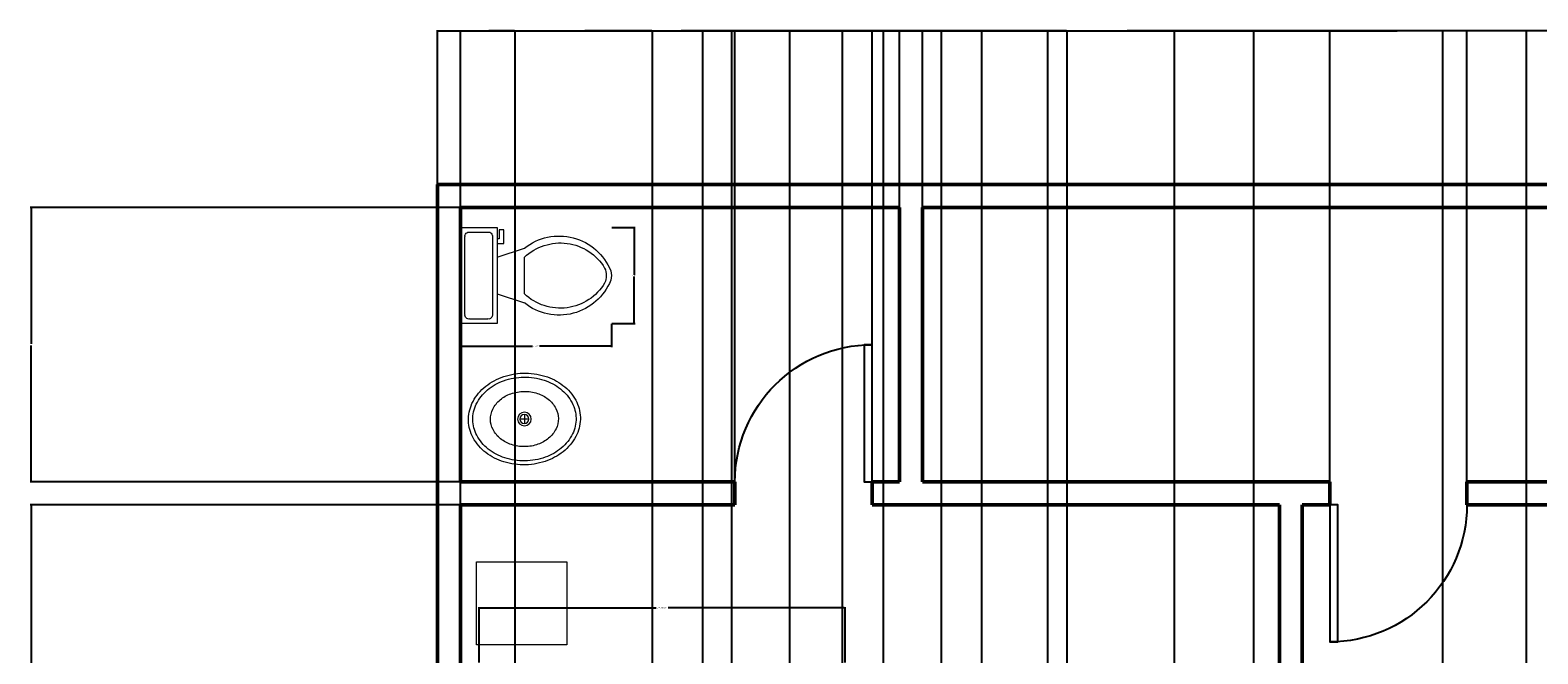
# Model space of a CAD drawing. Units: inches. Extents: x 115999 to 116502, y 188991 to 189729.
# Tile 4 of 5: x 115999 to 116329, y 189592 to 189729. Entities that reach past the tile are written whole.
import ezdxf

# ---------------------------------------------------------------- set-up
doc = ezdxf.new("R2010")
doc.units = ezdxf.units.IN
for name, color, linetype, lineweight in [('A-ANNO-DIMS', 2, 'Continuous', 18), ('A-DOOR', 4, 'Continuous', 25), ('A-FLOR-FIXT', 9, 'Continuous', 20), ('A-FURN', 8, 'Continuous', 18), ('A-WALL', 7, 'Continuous', 50)]:
    doc.layers.add(name, color=color, linetype=linetype, lineweight=lineweight)
doc.styles.get("Standard").update_dxf_attribs({"font": 'arial.ttf'})
doc.dimstyles.get("Standard").update_dxf_attribs({"dimtxt": 0.18, "dimasz": 0.18, "dimexe": 0.18, "dimexo": 0.0625, "dimgap": 0.09, "dimtad": 0, "dimtih": 1, "dimtoh": 1, "dimdec": 4, "dimzin": 0, "dimdsep": 46, "dimtxsty": 'Standard', "dimcen": 0.09, "dimadec": 0, "dimazin": 0, "dimtfac": 1, "dimtdec": 4, "dimtofl": 0, "dimtmove": 0, "dimatfit": 3, "dimfxl": 1, "dimtolj": 1, "dimtzin": 0, "dimarcsym": 0})

# ---------------------------------------------------------------- blocks, each defined once
blk = doc.blocks.new('*U3')
for p, q in [((0, 0), (0, -5)), ((30, 0), (30, -5))]:
    blk.add_line(p, q)
blk.add_lwpolyline([(0, 0), (0, 30), (1.75, 30), (1.75, 0)], close=True)
blk.add_arc((0, 0), 30, 0, 90)
blk = doc.blocks.new('Toilet - top')
for p, q in [((9.5, -6), (9.5, -2)), ((-10, -8.5), (-8, -8.5)), ((-10, -9.5), (-10, -8.5)), ((-7, -9.5), (-10, -9.5)), ((-8, -8.5), (-8, -8)), ((-7, -8), (-7, -9.5)), ((-4, -8), (-6, -14)), ((4, -8), (6, -14)), ((4, -14), (-4, -14))]:
    blk.add_line(p, q)
blk.add_lwpolyline([(10.5, -8), (10.5, 0), (-10.5, 0), (-10.5, -8)], close=True)
for points in [[(-9.5, -2), (-9.5, -6)], [(8.5, -1), (-8.5, -1)], [(-8.5, -7), (8.5, -7)]]:
    blk.add_lwpolyline(points)
for centre, radius, start, end in [((-8.62, -1.88), 0.884, 81.8699, 188.1301), ((8.62, -1.88), 0.884, 351.8699, 98.1301), ((-8.62, -6.12), 0.884, 171.8699, 278.1301), ((8.62, -6.12), 0.884, 261.8699, 8.1301), ((3.52, -21.58), 12.17, 141.4691, 247.9714), ((4.2, -21.82), 11.33, 136.3677, 238.9468), ((-3.52, -21.58), 12.17, 292.0284, 38.5307), ((-4.2, -21.82), 11.33, 301.053, 43.6321), ((0, -27.88), 4, 245.7318, 294.2682), ((0, -29), 4, 254.8605, 285.1395)]:
    blk.add_arc(centre, radius, start, end)
blk = doc.blocks.new('Sink - Oval top')
for p, q in [((-1, 0), (1, 0)), ((0, 1), (0, -1))]:
    blk.add_line(p, q)
for points in [[(-12.23, 0.39, 0.117634), (-11.46, -3.36, 0.104469), (-8.88, -6.8, 0.090016), (-5.08, -9.07, 0.08192), (-0.32, -10.02, 0.08192), (4.49, -9.38, 0.090016), (8.42, -7.36, 0.104469), (11.22, -4.09, 0.117634), (12.23, -0.39, 0.117634), (11.46, 3.36, 0.104469), (8.88, 6.8, 0.090016), (5.08, 9.07, 0.08192), (0.32, 10.02, 0.08192), (-4.49, 9.38, 0.090016), (-8.42, 7.36, 0.104469), (-11.22, 4.09, 0.117634)], [(-11.29, 0.16, 0.118622), (-10.52, -3.25, 0.104678), (-8.07, -6.36, 0.089562), (-4.54, -8.37, 0.081185), (-0.13, -9.15, 0.081185), (4.3, -8.49, 0.089562), (7.89, -6.58, 0.104678), (10.42, -3.55, 0.118622), (11.29, -0.16, 0.118622), (10.52, 3.25, 0.104678), (8.07, 6.36, 0.089562), (4.54, 8.37, 0.081185), (0.13, 9.15, 0.081185), (-4.3, 8.49, 0.089562), (-7.89, 6.58, 0.104678), (-10.42, 3.55, 0.118622)], [(-7.42, 0.08, 0.118283), (-6.91, -2.17, 0.104607), (-5.29, -4.21, 0.089718), (-2.97, -5.53, 0.081436), (-0.07, -6.04, 0.081436), (2.84, -5.59, 0.089718), (5.2, -4.33, 0.104607), (6.86, -2.32, 0.118283), (7.42, -0.08, 0.118283), (6.91, 2.17, 0.104607), (5.29, 4.21, 0.089718), (2.97, 5.53, 0.081436), (0.07, 6.04, 0.081436), (-2.84, 5.59, 0.089718), (-5.2, 4.33, 0.104607), (-6.86, 2.32, 0.118283)]]:
    blk.add_lwpolyline(points, format="xyb", close=True)
for radius in [1.5, 1]:
    blk.add_circle((0, 0), radius)
blk = doc.blocks.new('TABLE-NIGHTSTAND')
blk.add_lwpolyline([(0, 18.2), (19.71, 18.2), (19.71, 0), (0, 0)], close=True)
blk = doc.blocks.new('*D19')
at = {"layer": 'A-ANNO-DIMS', "color": 0, "lineweight": -2, "transparency": 16777216}
for p, q in [((116093.06, 189664.5), (116093.06, 189659.43)), ((116126.11, 189664.5), (116126.11, 189659.43)), ((116093.24, 189659.61), (116108.81, 189659.61)), ((116125.93, 189659.61), (116110.36, 189659.61))]:
    blk.add_line(p, q, dxfattribs=at)
at = {"layer": 'A-ANNO-DIMS', "color": 0, "transparency": 16777216}
for points in [[(116093.24, 189659.64), (116093.24, 189659.58), (116093.06, 189659.61)], [(116125.93, 189659.64), (116125.93, 189659.58), (116126.11, 189659.61)]]:
    blk.add_solid(points, dxfattribs=at)
at = {"layer": 'Defpoints', "color": 0, "transparency": 16777216}
for p in [(116093.06, 189664.57), (116126.11, 189664.57), (116093.06, 189659.61)]:
    blk.add_point(p, dxfattribs=at)
at = {"layer": 'A-ANNO-DIMS', "color": 0, "transparency": 16777216, "insert": (116109.59, 189659.61), "char_height": 0.18, "attachment_point": 5}
blk.add_mtext('\\A1;WC 33 TYP.', dxfattribs=at)
blk = doc.blocks.new('*D20')
at = {"layer": 'A-ANNO-DIMS', "color": 0, "lineweight": -2, "transparency": 16777216}
for p, q in [((116126.17, 189685.57), (116131.25, 189685.57)), ((116131.07, 189685.39), (116131.07, 189675.25)), ((116131.07, 189664.75), (116131.07, 189674.89)), ((116126.17, 189664.57), (116131.25, 189664.57))]:
    blk.add_line(p, q, dxfattribs=at)
at = {"layer": 'A-ANNO-DIMS', "color": 0, "transparency": 16777216}
for points in [[(116131.04, 189685.39), (116131.1, 189685.39), (116131.07, 189685.57)], [(116131.04, 189664.75), (116131.1, 189664.75), (116131.07, 189664.57)]]:
    blk.add_solid(points, dxfattribs=at)
at = {"layer": 'Defpoints', "color": 0, "transparency": 16777216}
for p in [(116126.11, 189685.57), (116126.11, 189664.57), (116131.07, 189664.57)]:
    blk.add_point(p, dxfattribs=at)
at = {"layer": 'A-ANNO-DIMS', "color": 0, "transparency": 16777216, "insert": (116131.07, 189675.07), "char_height": 0.18, "attachment_point": 5}
blk.add_mtext('\\A1;21 TYP.', dxfattribs=at)
blk = doc.blocks.new('*D21')
at = {"layer": 'A-ANNO-DIMS', "color": 0, "lineweight": -2, "transparency": 16777216}
for p, q in [((116097.14, 189590.46), (116097.14, 189602.58)), ((116097.32, 189602.4), (116135.84, 189602.4)), ((116176.96, 189602.4), (116138.45, 189602.4)), ((116177.14, 189590.46), (116177.14, 189602.58))]:
    blk.add_line(p, q, dxfattribs=at)
at = {"layer": 'A-ANNO-DIMS', "color": 0, "transparency": 16777216}
for points in [[(116097.32, 189602.43), (116097.32, 189602.37), (116097.14, 189602.4)], [(116176.96, 189602.43), (116176.96, 189602.37), (116177.14, 189602.4)]]:
    blk.add_solid(points, dxfattribs=at)
at = {"layer": 'Defpoints', "color": 0, "transparency": 16777216}
for p in [(116097.14, 189602.4), (116097.14, 189590.4), (116177.14, 189590.4)]:
    blk.add_point(p, dxfattribs=at)
at = {"layer": 'A-ANNO-DIMS', "color": 0, "transparency": 16777216, "insert": (116137.14, 189602.4), "char_height": 0.18, "attachment_point": 5}
blk.add_mtext('\\A1;QUEEN BED 80 TYP.', dxfattribs=at)
blk = doc.blocks.new('*D33')
at = {"layer": 'A-ANNO-DIMS', "color": 0, "lineweight": -2, "transparency": 16777216}
for p, q in [((116088.06, 189088.01), (116088.06, 189728.73)), ((116088.24, 189728.55), (116277.77, 189728.55)), ((116467.88, 189728.55), (116278.35, 189728.55)), ((116468.06, 189088.01), (116468.06, 189728.73))]:
    blk.add_line(p, q, dxfattribs=at)
at = {"layer": 'A-ANNO-DIMS', "color": 0, "transparency": 16777216}
for points in [[(116088.24, 189728.58), (116088.24, 189728.52), (116088.06, 189728.55)], [(116467.88, 189728.58), (116467.88, 189728.52), (116468.06, 189728.55)]]:
    blk.add_solid(points, dxfattribs=at)
at = {"layer": 'Defpoints', "color": 0, "transparency": 16777216}
for p in [(116468.06, 189728.55), (116088.06, 189087.95), (116468.06, 189087.95)]:
    blk.add_point(p, dxfattribs=at)
at = {"layer": 'A-ANNO-DIMS', "color": 0, "transparency": 16777216, "insert": (116278.06, 189728.55), "char_height": 0.18, "attachment_point": 5}
blk.add_mtext('\\A1;380', dxfattribs=at)
blk = doc.blocks.new('*D35')
at = {"layer": 'A-ANNO-DIMS', "color": 0, "lineweight": -2, "transparency": 16777216}
for p, q in [((116093.06, 189690.01), (116093.06, 189728.73)), ((116093.24, 189728.55), (116140.84, 189728.55)), ((116188.88, 189728.55), (116141.28, 189728.55)), ((116189.06, 189690.01), (116189.06, 189728.73))]:
    blk.add_line(p, q, dxfattribs=at)
at = {"layer": 'A-ANNO-DIMS', "color": 0, "transparency": 16777216}
for points in [[(116093.24, 189728.58), (116093.24, 189728.52), (116093.06, 189728.55)], [(116188.88, 189728.58), (116188.88, 189728.52), (116189.06, 189728.55)]]:
    blk.add_solid(points, dxfattribs=at)
at = {"layer": 'Defpoints', "color": 0, "transparency": 16777216}
for p in [(116189.06, 189728.55), (116093.06, 189689.95), (116189.06, 189689.95)]:
    blk.add_point(p, dxfattribs=at)
at = {"layer": 'A-ANNO-DIMS', "color": 0, "transparency": 16777216, "insert": (116141.06, 189728.55), "char_height": 0.18, "attachment_point": 5}
blk.add_mtext('\\A1;96', dxfattribs=at)
blk = doc.blocks.new('*D36')
at = {"layer": 'A-ANNO-DIMS', "color": 0, "lineweight": -2, "transparency": 16777216}
for p, q in [((116194.06, 189690.01), (116194.06, 189728.73)), ((116194.24, 189728.55), (116277.78, 189728.55)), ((116361.88, 189728.55), (116278.34, 189728.55)), ((116362.06, 189690.01), (116362.06, 189728.73))]:
    blk.add_line(p, q, dxfattribs=at)
at = {"layer": 'A-ANNO-DIMS', "color": 0, "transparency": 16777216}
for points in [[(116194.24, 189728.58), (116194.24, 189728.52), (116194.06, 189728.55)], [(116361.88, 189728.58), (116361.88, 189728.52), (116362.06, 189728.55)]]:
    blk.add_solid(points, dxfattribs=at)
at = {"layer": 'Defpoints', "color": 0, "transparency": 16777216}
for p in [(116362.06, 189728.55), (116194.06, 189689.95), (116362.06, 189689.95)]:
    blk.add_point(p, dxfattribs=at)
at = {"layer": 'A-ANNO-DIMS', "color": 0, "transparency": 16777216, "insert": (116278.06, 189728.55), "char_height": 0.18, "attachment_point": 5}
blk.add_mtext('\\A1;168', dxfattribs=at)
blk = doc.blocks.new('*D38')
at = {"layer": 'A-ANNO-DIMS', "color": 0, "lineweight": -2, "transparency": 16777216}
for p, q in [((116093, 189689.95), (115999.04, 189689.95)), ((115999.22, 189689.77), (115999.22, 189660.13)), ((115999.22, 189630.13), (115999.22, 189659.77)), ((116093, 189629.95), (115999.04, 189629.95))]:
    blk.add_line(p, q, dxfattribs=at)
at = {"layer": 'A-ANNO-DIMS', "color": 0, "transparency": 16777216}
for points in [[(115999.19, 189689.77), (115999.25, 189689.77), (115999.22, 189689.95)], [(115999.19, 189630.13), (115999.25, 189630.13), (115999.22, 189629.95)]]:
    blk.add_solid(points, dxfattribs=at)
at = {"layer": 'Defpoints', "color": 0, "transparency": 16777216}
for p in [(115999.22, 189689.95), (116093.06, 189689.95), (116093.06, 189629.95)]:
    blk.add_point(p, dxfattribs=at)
at = {"layer": 'A-ANNO-DIMS', "color": 0, "transparency": 16777216, "insert": (115999.22, 189659.95), "char_height": 0.18, "attachment_point": 5}
blk.add_mtext('\\A1;60', dxfattribs=at)
blk = doc.blocks.new('*D39')
at = {"layer": 'A-ANNO-DIMS', "color": 0, "lineweight": -2, "transparency": 16777216}
for p, q in [((116093, 189624.95), (115999.04, 189624.95)), ((115999.22, 189624.77), (115999.22, 189556.13)), ((115999.22, 189487.13), (115999.22, 189555.76)), ((116093, 189486.95), (115999.04, 189486.95))]:
    blk.add_line(p, q, dxfattribs=at)
at = {"layer": 'A-ANNO-DIMS', "color": 0, "transparency": 16777216}
for points in [[(115999.19, 189624.77), (115999.25, 189624.77), (115999.22, 189624.95)], [(115999.19, 189487.13), (115999.25, 189487.13), (115999.22, 189486.95)]]:
    blk.add_solid(points, dxfattribs=at)
at = {"layer": 'Defpoints', "color": 0, "transparency": 16777216}
for p in [(115999.22, 189624.95), (116093.06, 189624.95), (116093.06, 189486.95)]:
    blk.add_point(p, dxfattribs=at)
at = {"layer": 'A-ANNO-DIMS', "color": 0, "transparency": 16777216, "insert": (115999.22, 189555.95), "char_height": 0.18, "attachment_point": 5}
blk.add_mtext('\\A1;138', dxfattribs=at)
blk = doc.blocks.new('*D43')
at = {"layer": 'A-ANNO-DIMS', "color": 0, "lineweight": -2, "transparency": 16777216}
for p, q in [((116093.06, 189624.88), (116093.06, 188991.26)), ((116272.06, 189624.88), (116272.06, 188991.26)), ((116093.24, 188991.44), (116182.28, 188991.44)), ((116271.88, 188991.44), (116182.84, 188991.44))]:
    blk.add_line(p, q, dxfattribs=at)
at = {"layer": 'A-ANNO-DIMS', "color": 0, "transparency": 16777216}
for points in [[(116093.24, 188991.47), (116093.24, 188991.41), (116093.06, 188991.44)], [(116271.88, 188991.47), (116271.88, 188991.41), (116272.06, 188991.44)]]:
    blk.add_solid(points, dxfattribs=at)
at = {"layer": 'Defpoints', "color": 0, "transparency": 16777216}
for p in [(116093.06, 189624.95), (116272.06, 189624.95), (116272.06, 188991.44)]:
    blk.add_point(p, dxfattribs=at)
at = {"layer": 'A-ANNO-DIMS', "color": 0, "transparency": 16777216, "insert": (116182.56, 188991.44), "char_height": 0.18, "attachment_point": 5}
blk.add_mtext('\\A1;179', dxfattribs=at)
blk = doc.blocks.new('*D44')
at = {"layer": 'A-ANNO-DIMS', "color": 0, "lineweight": -2, "transparency": 16777216}
for p, q in [((116277.06, 189624.88), (116277.06, 188991.26)), ((116463.06, 189624.88), (116463.06, 188991.26)), ((116277.24, 188991.44), (116369.78, 188991.44)), ((116462.88, 188991.44), (116370.34, 188991.44))]:
    blk.add_line(p, q, dxfattribs=at)
at = {"layer": 'A-ANNO-DIMS', "color": 0, "transparency": 16777216}
for points in [[(116277.24, 188991.47), (116277.24, 188991.41), (116277.06, 188991.44)], [(116462.88, 188991.47), (116462.88, 188991.41), (116463.06, 188991.44)]]:
    blk.add_solid(points, dxfattribs=at)
at = {"layer": 'Defpoints', "color": 0, "transparency": 16777216}
for p in [(116277.06, 189624.95), (116463.06, 189624.95), (116463.06, 188991.44)]:
    blk.add_point(p, dxfattribs=at)
at = {"layer": 'A-ANNO-DIMS', "color": 0, "transparency": 16777216, "insert": (116370.06, 188991.44), "char_height": 0.18, "attachment_point": 5}
blk.add_mtext('\\A1;186', dxfattribs=at)
blk = doc.blocks.new('*D45')
at = {"layer": 'A-ANNO-DIMS', "color": 0, "lineweight": -2, "transparency": 16777216}
for p, q in [((116272.06, 189624.88), (116272.06, 188991.26)), ((116277.06, 189624.88), (116277.06, 188991.26)), ((116272.24, 188991.44), (116274.41, 188991.44)), ((116276.88, 188991.44), (116274.71, 188991.44))]:
    blk.add_line(p, q, dxfattribs=at)
at = {"layer": 'A-ANNO-DIMS', "color": 0, "transparency": 16777216}
for points in [[(116272.24, 188991.47), (116272.24, 188991.41), (116272.06, 188991.44)], [(116276.88, 188991.47), (116276.88, 188991.41), (116277.06, 188991.44)]]:
    blk.add_solid(points, dxfattribs=at)
at = {"layer": 'Defpoints', "color": 0, "transparency": 16777216}
for p in [(116272.06, 189624.95), (116277.06, 189624.95), (116277.06, 188991.44)]:
    blk.add_point(p, dxfattribs=at)
at = {"layer": 'A-ANNO-DIMS', "color": 0, "transparency": 16777216, "insert": (116274.56, 188991.44), "char_height": 0.18, "attachment_point": 5}
blk.add_mtext('\\A1;5', dxfattribs=at)
blk = doc.blocks.new('*D48')
at = {"layer": 'A-ANNO-DIMS', "color": 0, "lineweight": -2, "transparency": 16777216}
for p, q in [((116153.06, 189630.01), (116153.06, 189728.73)), ((116153.24, 189728.55), (116167.84, 189728.55)), ((116182.88, 189728.55), (116168.28, 189728.55)), ((116183.06, 189630.01), (116183.06, 189728.73))]:
    blk.add_line(p, q, dxfattribs=at)
at = {"layer": 'A-ANNO-DIMS', "color": 0, "transparency": 16777216}
for points in [[(116153.24, 189728.58), (116153.24, 189728.52), (116153.06, 189728.55)], [(116182.88, 189728.58), (116182.88, 189728.52), (116183.06, 189728.55)]]:
    blk.add_solid(points, dxfattribs=at)
at = {"layer": 'Defpoints', "color": 0, "transparency": 16777216}
for p in [(116183.06, 189728.55), (116153.06, 189629.95), (116183.06, 189629.95)]:
    blk.add_point(p, dxfattribs=at)
at = {"layer": 'A-ANNO-DIMS', "color": 0, "transparency": 16777216, "insert": (116168.06, 189728.55), "char_height": 0.18, "attachment_point": 5}
blk.add_mtext('\\A1;30', dxfattribs=at)
blk = doc.blocks.new('*D54')
at = {"layer": 'A-ANNO-DIMS', "color": 0, "lineweight": -2, "transparency": 16777216}
for p, q in [((116266.5, 189437.51), (116266.5, 189728.73)), ((116266.68, 189728.55), (116286.73, 189728.55)), ((116307.58, 189728.55), (116287.53, 189728.55)), ((116307.76, 189437.51), (116307.76, 189728.73))]:
    blk.add_line(p, q, dxfattribs=at)
at = {"layer": 'A-ANNO-DIMS', "color": 0, "transparency": 16777216}
for points in [[(116266.68, 189728.58), (116266.68, 189728.52), (116266.5, 189728.55)], [(116307.58, 189728.58), (116307.58, 189728.52), (116307.76, 189728.55)]]:
    blk.add_solid(points, dxfattribs=at)
at = {"layer": 'Defpoints', "color": 0, "transparency": 16777216}
for p in [(116307.76, 189728.55), (116266.5, 189437.45), (116307.76, 189437.45)]:
    blk.add_point(p, dxfattribs=at)
at = {"layer": 'A-ANNO-DIMS', "color": 0, "transparency": 16777216, "insert": (116287.13, 189728.55), "char_height": 0.18, "attachment_point": 5}
blk.add_mtext('\\A1;41.26', dxfattribs=at)
blk = doc.blocks.new('*D70')
at = {"layer": 'A-ANNO-DIMS', "color": 0, "lineweight": -2, "transparency": 16777216}
for p, q in [((116105.06, 189350.01), (116105.06, 189728.73)), ((116105.24, 189728.55), (116119.84, 189728.55)), ((116134.88, 189728.55), (116120.28, 189728.55)), ((116135.06, 189350.01), (116135.06, 189728.73))]:
    blk.add_line(p, q, dxfattribs=at)
at = {"layer": 'A-ANNO-DIMS', "color": 0, "transparency": 16777216}
for points in [[(116105.24, 189728.58), (116105.24, 189728.52), (116105.06, 189728.55)], [(116134.88, 189728.58), (116134.88, 189728.52), (116135.06, 189728.55)]]:
    blk.add_solid(points, dxfattribs=at)
at = {"layer": 'Defpoints', "color": 0, "transparency": 16777216}
for p in [(116135.06, 189728.55), (116105.06, 189349.95), (116135.06, 189349.95)]:
    blk.add_point(p, dxfattribs=at)
at = {"layer": 'A-ANNO-DIMS', "color": 0, "transparency": 16777216, "insert": (116120.06, 189728.55), "char_height": 0.18, "attachment_point": 5}
blk.add_mtext('\\A1;30', dxfattribs=at)
blk = doc.blocks.new('*D71')
at = {"layer": 'A-ANNO-DIMS', "color": 0, "lineweight": -2, "transparency": 16777216}
for p, q in [((116165.06, 189350.01), (116165.06, 189728.73)), ((116165.24, 189728.55), (116185.84, 189728.55)), ((116206.88, 189728.55), (116186.28, 189728.55)), ((116207.06, 189350.01), (116207.06, 189728.73))]:
    blk.add_line(p, q, dxfattribs=at)
at = {"layer": 'A-ANNO-DIMS', "color": 0, "transparency": 16777216}
for points in [[(116165.24, 189728.58), (116165.24, 189728.52), (116165.06, 189728.55)], [(116206.88, 189728.58), (116206.88, 189728.52), (116207.06, 189728.55)]]:
    blk.add_solid(points, dxfattribs=at)
at = {"layer": 'Defpoints', "color": 0, "transparency": 16777216}
for p in [(116207.06, 189728.55), (116165.06, 189349.95), (116207.06, 189349.95)]:
    blk.add_point(p, dxfattribs=at)
at = {"layer": 'A-ANNO-DIMS', "color": 0, "transparency": 16777216, "insert": (116186.06, 189728.55), "char_height": 0.18, "attachment_point": 5}
blk.add_mtext('\\A1;42', dxfattribs=at)
blk = doc.blocks.new('*D72')
at = {"layer": 'A-ANNO-DIMS', "color": 0, "lineweight": -2, "transparency": 16777216}
for p, q in [((116249.18, 189350.01), (116249.18, 189728.73)), ((116249.36, 189728.55), (116287.23, 189728.55)), ((116325.88, 189728.55), (116288.02, 189728.55)), ((116326.06, 189350.01), (116326.06, 189728.73))]:
    blk.add_line(p, q, dxfattribs=at)
at = {"layer": 'A-ANNO-DIMS', "color": 0, "transparency": 16777216}
for points in [[(116249.36, 189728.58), (116249.36, 189728.52), (116249.18, 189728.55)], [(116325.88, 189728.58), (116325.88, 189728.52), (116326.06, 189728.55)]]:
    blk.add_solid(points, dxfattribs=at)
at = {"layer": 'Defpoints', "color": 0, "transparency": 16777216}
for p in [(116326.06, 189728.55), (116249.18, 189349.95), (116326.06, 189349.95)]:
    blk.add_point(p, dxfattribs=at)
at = {"layer": 'A-ANNO-DIMS', "color": 0, "transparency": 16777216, "insert": (116287.62, 189728.55), "char_height": 0.18, "attachment_point": 5}
blk.add_mtext('\\A1;76.88', dxfattribs=at)
blk = doc.blocks.new('*D73')
at = {"layer": 'A-ANNO-DIMS', "color": 0, "lineweight": -2, "transparency": 16777216}
for p, q in [((116093.06, 189350.01), (116093.06, 189728.73)), ((116093.24, 189728.55), (116098.85, 189728.55)), ((116104.88, 189728.55), (116099.27, 189728.55)), ((116105.06, 189350.01), (116105.06, 189728.73))]:
    blk.add_line(p, q, dxfattribs=at)
at = {"layer": 'A-ANNO-DIMS', "color": 0, "transparency": 16777216}
for points in [[(116093.24, 189728.58), (116093.24, 189728.52), (116093.06, 189728.55)], [(116104.88, 189728.58), (116104.88, 189728.52), (116105.06, 189728.55)]]:
    blk.add_solid(points, dxfattribs=at)
at = {"layer": 'Defpoints', "color": 0, "transparency": 16777216}
for p in [(116105.06, 189728.55), (116093.06, 189349.95), (116105.06, 189349.95)]:
    blk.add_point(p, dxfattribs=at)
at = {"layer": 'A-ANNO-DIMS', "color": 0, "transparency": 16777216, "insert": (116099.06, 189728.55), "char_height": 0.18, "attachment_point": 5}
blk.add_mtext('\\A1;12', dxfattribs=at)
blk = doc.blocks.new('*D74')
at = {"layer": 'A-ANNO-DIMS', "color": 0, "lineweight": -2, "transparency": 16777216}
for p, q in [((116146.06, 189350.01), (116146.06, 189728.73)), ((116146.24, 189728.55), (116155.35, 189728.55)), ((116164.88, 189728.55), (116155.77, 189728.55)), ((116165.06, 189350.01), (116165.06, 189728.73))]:
    blk.add_line(p, q, dxfattribs=at)
at = {"layer": 'A-ANNO-DIMS', "color": 0, "transparency": 16777216}
for points in [[(116146.24, 189728.58), (116146.24, 189728.52), (116146.06, 189728.55)], [(116164.88, 189728.58), (116164.88, 189728.52), (116165.06, 189728.55)]]:
    blk.add_solid(points, dxfattribs=at)
at = {"layer": 'Defpoints', "color": 0, "transparency": 16777216}
for p in [(116165.06, 189728.55), (116146.06, 189349.95), (116165.06, 189349.95)]:
    blk.add_point(p, dxfattribs=at)
at = {"layer": 'A-ANNO-DIMS', "color": 0, "transparency": 16777216, "insert": (116155.56, 189728.55), "char_height": 0.18, "attachment_point": 5}
blk.add_mtext('\\A1;19', dxfattribs=at)
blk = doc.blocks.new('*D75')
at = {"layer": 'A-ANNO-DIMS', "color": 0, "lineweight": -2, "transparency": 16777216}
for p, q in [((116183.063078, 189630.009428), (116183.063078, 189728.726928)), ((116183.243078, 189728.546928), (116185.913651, 189728.546928)), ((116188.883078, 189728.546928), (116186.212505, 189728.546928)), ((116189.063078, 189630.009428), (116189.063078, 189728.726928))]:
    blk.add_line(p, q, dxfattribs=at)
at = {"layer": 'A-ANNO-DIMS', "color": 0, "transparency": 16777216}
for points in [[(116183.243078, 189728.576928), (116183.243078, 189728.516928), (116183.063078, 189728.546928)], [(116188.883078, 189728.576928), (116188.883078, 189728.516928), (116189.063078, 189728.546928)]]:
    blk.add_solid(points, dxfattribs=at)
at = {"layer": 'Defpoints', "color": 0, "transparency": 16777216}
for p in [(116189.063078, 189728.546928), (116183.063078, 189629.946928), (116189.063078, 189629.946928)]:
    blk.add_point(p, dxfattribs=at)
at = {"layer": 'A-ANNO-DIMS', "color": 0, "transparency": 16777216, "insert": (116186.063078, 189728.546928), "char_height": 0.18, "attachment_point": 5}
blk.add_mtext('\\A1;6', dxfattribs=at)
blk = doc.blocks.new('*D76')
at = {"layer": 'A-ANNO-DIMS', "color": 0, "lineweight": -2, "transparency": 16777216}
for p, q in [((116194.06, 189630.01), (116194.06, 189728.73)), ((116194.24, 189728.55), (116238.34, 189728.55)), ((116282.88, 189728.55), (116238.78, 189728.55)), ((116283.06, 189630.01), (116283.06, 189728.73))]:
    blk.add_line(p, q, dxfattribs=at)
at = {"layer": 'A-ANNO-DIMS', "color": 0, "transparency": 16777216}
for points in [[(116194.24, 189728.58), (116194.24, 189728.52), (116194.06, 189728.55)], [(116282.88, 189728.58), (116282.88, 189728.52), (116283.06, 189728.55)]]:
    blk.add_solid(points, dxfattribs=at)
at = {"layer": 'Defpoints', "color": 0, "transparency": 16777216}
for p in [(116283.06, 189728.55), (116194.06, 189629.95), (116283.06, 189629.95)]:
    blk.add_point(p, dxfattribs=at)
at = {"layer": 'A-ANNO-DIMS', "color": 0, "transparency": 16777216, "insert": (116238.56, 189728.55), "char_height": 0.18, "attachment_point": 5}
blk.add_mtext('\\A1;89', dxfattribs=at)
blk = doc.blocks.new('*D77')
at = {"layer": 'A-ANNO-DIMS', "color": 0, "lineweight": -2, "transparency": 16777216}
for p, q in [((116283.06, 189630.01), (116283.06, 189728.73)), ((116283.24, 189728.55), (116297.84, 189728.55)), ((116312.88, 189728.55), (116298.28, 189728.55)), ((116313.06, 189630.01), (116313.06, 189728.73))]:
    blk.add_line(p, q, dxfattribs=at)
at = {"layer": 'A-ANNO-DIMS', "color": 0, "transparency": 16777216}
for points in [[(116283.24, 189728.58), (116283.24, 189728.52), (116283.06, 189728.55)], [(116312.88, 189728.58), (116312.88, 189728.52), (116313.06, 189728.55)]]:
    blk.add_solid(points, dxfattribs=at)
at = {"layer": 'Defpoints', "color": 0, "transparency": 16777216}
for p in [(116313.06, 189728.55), (116283.06, 189629.95), (116313.06, 189629.95)]:
    blk.add_point(p, dxfattribs=at)
at = {"layer": 'A-ANNO-DIMS', "color": 0, "transparency": 16777216, "insert": (116298.06, 189728.55), "char_height": 0.18, "attachment_point": 5}
blk.add_mtext('\\A1;30', dxfattribs=at)
blk = doc.blocks.new('*D78')
at = {"layer": 'A-ANNO-DIMS', "color": 0, "lineweight": -2, "transparency": 16777216}
for p, q in [((116198.25, 189429.74), (116198.25, 189728.73)), ((116198.43, 189728.55), (116209.47, 189728.55)), ((116221.29, 189728.55), (116210.25, 189728.55)), ((116221.47, 189429.74), (116221.47, 189728.73))]:
    blk.add_line(p, q, dxfattribs=at)
at = {"layer": 'A-ANNO-DIMS', "color": 0, "transparency": 16777216}
for points in [[(116198.43, 189728.58), (116198.43, 189728.52), (116198.25, 189728.55)], [(116221.29, 189728.58), (116221.29, 189728.52), (116221.47, 189728.55)]]:
    blk.add_solid(points, dxfattribs=at)
at = {"layer": 'Defpoints', "color": 0, "transparency": 16777216}
for p in [(116221.47, 189728.55), (116198.25, 189429.68), (116221.47, 189429.68)]:
    blk.add_point(p, dxfattribs=at)
at = {"layer": 'A-ANNO-DIMS', "color": 0, "transparency": 16777216, "insert": (116209.86, 189728.55), "char_height": 0.18, "attachment_point": 5}
blk.add_mtext('\\A1;23.22', dxfattribs=at)
blk = doc.blocks.new('*D80')
at = {"layer": 'A-ANNO-DIMS', "color": 0, "lineweight": -2, "transparency": 16777216}
for p, q in [((116185.52, 189476.05), (116185.52, 189728.73)), ((116185.7, 189728.55), (116205.21, 189728.55)), ((116225.51, 189728.55), (116206, 189728.55)), ((116225.69, 189476.05), (116225.69, 189728.73))]:
    blk.add_line(p, q, dxfattribs=at)
at = {"layer": 'A-ANNO-DIMS', "color": 0, "transparency": 16777216}
for points in [[(116185.7, 189728.58), (116185.7, 189728.52), (116185.52, 189728.55)], [(116225.51, 189728.58), (116225.51, 189728.52), (116225.69, 189728.55)]]:
    blk.add_solid(points, dxfattribs=at)
at = {"layer": 'Defpoints', "color": 0, "transparency": 16777216}
for p in [(116225.69, 189728.55), (116185.52, 189475.99), (116225.69, 189475.99)]:
    blk.add_point(p, dxfattribs=at)
at = {"layer": 'A-ANNO-DIMS', "color": 0, "transparency": 16777216, "insert": (116205.6, 189728.55), "char_height": 0.18, "attachment_point": 5}
blk.add_mtext('\\A1;40.17', dxfattribs=at)
blk = doc.blocks.new('*D82')
at = {"layer": 'A-ANNO-DIMS', "color": 0, "lineweight": -2, "transparency": 16777216}
for p, q in [((116152.4, 189477.27), (116152.4, 189728.73)), ((116152.58, 189728.55), (116164.04, 189728.55)), ((116176.43, 189728.55), (116164.97, 189728.55)), ((116176.61, 189477.27), (116176.61, 189728.73))]:
    blk.add_line(p, q, dxfattribs=at)
at = {"layer": 'A-ANNO-DIMS', "color": 0, "transparency": 16777216}
for points in [[(116152.58, 189728.58), (116152.58, 189728.52), (116152.4, 189728.55)], [(116176.43, 189728.58), (116176.43, 189728.52), (116176.61, 189728.55)]]:
    blk.add_solid(points, dxfattribs=at)
at = {"layer": 'Defpoints', "color": 0, "transparency": 16777216}
for p in [(116176.61, 189728.55), (116152.4, 189477.21), (116176.61, 189477.21)]:
    blk.add_point(p, dxfattribs=at)
at = {"layer": 'A-ANNO-DIMS', "color": 0, "transparency": 16777216, "insert": (116164.51, 189728.55), "char_height": 0.18, "attachment_point": 5}
blk.add_mtext('\\A1;24.204', dxfattribs=at)

msp = doc.modelspace()

# ---------------------------------------------------------------- linework, layer by layer
at = {"layer": 'A-WALL'}
for p, q in [((116088.0631, 189694.9469), (116468.0631, 189694.9469)), ((116088.0631, 189694.9469), (116088.0631, 189087.9469)), ((116093.0631, 189689.9469), (116189.0631, 189689.9469)), ((116093.0631, 189689.9469), (116093.0631, 189629.9469)), ((116189.0631, 189689.9469), (116189.0631, 189629.9469)), ((116194.0631, 189689.9469), (116194.0631, 189629.9469)), ((116194.0631, 189689.9469), (116362.0631, 189689.9469)), ((116093.0631, 189629.9469), (116153.0631, 189629.9469)), ((116153.0631, 189629.9469), (116153.0631, 189624.9469)), ((116183.0631, 189629.9469), (116183.0631, 189624.9469)), ((116183.0631, 189629.9469), (116189.0631, 189629.9469)), ((116194.0631, 189629.9469), (116283.0631, 189629.9469)), ((116283.0631, 189624.9469), (116283.0631, 189629.9469)), ((116313.0631, 189624.9469), (116313.0631, 189629.9469)), ((116313.0631, 189629.9469), (116362.0631, 189629.9469)), ((116093.0631, 189624.9469), (116153.0631, 189624.9469)), ((116093.0631, 189624.9469), (116093.0631, 189486.9469)), ((116183.0631, 189624.9469), (116272.0631, 189624.9469)), ((116272.0631, 189624.9469), (116272.0631, 189486.9469)), ((116277.0631, 189624.9469), (116277.0631, 189486.9469)), ((116277.0631, 189624.9469), (116283.0631, 189624.9469)), ((116313.0631, 189624.9469), (116373.0631, 189624.9469))]:
    msp.add_line(p, q, dxfattribs=at)

# ---------------------------------------------------------------- block references
at = {"layer": 'A-DOOR', "xscale": -1}
msp.add_blockref('*U3', (116183.0631, 189629.9469), dxfattribs=at)
at = {"layer": 'A-DOOR', "xscale": -1, "rotation": 180}
msp.add_blockref('*U3', (116283.0631, 189624.9469), dxfattribs=at)
at = {"layer": 'A-FLOR-FIXT', "xscale": -1, "rotation": 90}
msp.add_blockref('Toilet - top', (116093.0631, 189675.0657), dxfattribs=at)
at = {"layer": 'A-FLOR-FIXT', "xscale": -1}
msp.add_blockref('Sink - Oval top', (116107.0496, 189643.6992), dxfattribs=at)
at = {"layer": 'A-FURN'}
msp.add_blockref('TABLE-NIGHTSTAND', (116096.5803, 189594.2971), dxfattribs=at)

# ---------------------------------------------------------------- dimensions: what is measured, and where the dimension line sits
at = {"layer": 'A-ANNO-DIMS'}
for base, p1, p2, override, picture, middle in [((116468.0631, 189728.5469), (116088.0631, 189087.9469), (116468.0631, 189087.9469), {"dimdec": 0, "dimlfac": 1, "dimrnd": 0, "dimzin": 0, "dimdsep": 46, "dimlunit": 2}, '*D33', (116278.0631, 189728.5469)), ((116189.0631, 189728.5469), (116093.0631, 189689.9469), (116189.0631, 189689.9469), {"dimdec": 0, "dimlfac": 1, "dimrnd": 0, "dimzin": 0, "dimdsep": 46, "dimlunit": 2}, '*D35', (116141.0631, 189728.5469)), ((116105.0631, 189728.5469), (116093.0631, 189349.9469), (116105.0631, 189349.9469), {"dimdec": 0, "dimlfac": 1, "dimrnd": 0, "dimzin": 0, "dimdsep": 46, "dimlunit": 2}, '*D73', (116099.0631, 189728.5469)), ((116135.0631, 189728.5469), (116105.0631, 189349.9469), (116135.0631, 189349.9469), {"dimdec": 0, "dimlfac": 1, "dimrnd": 0, "dimzin": 0, "dimdsep": 46, "dimlunit": 2}, '*D70', (116120.0631, 189728.5469)), ((116165.0631, 189728.5469), (116146.0631, 189349.9469), (116165.0631, 189349.9469), {"dimdec": 0, "dimlfac": 1, "dimrnd": 0, "dimzin": 0, "dimdsep": 46, "dimlunit": 2}, '*D74', (116155.5631, 189728.5469)), ((116176.6085, 189728.5469), (116152.4048, 189477.2058), (116176.6085, 189477.2058), {"dimdec": 3, "dimlfac": 1, "dimrnd": 0, "dimzin": 0, "dimdsep": 46, "dimlunit": 2}, '*D82', (116164.5066, 189728.5469)), ((116183.0631, 189728.5469), (116153.0631, 189629.9469), (116183.0631, 189629.9469), {"dimdec": 0, "dimlfac": 1, "dimrnd": 0, "dimzin": 0, "dimdsep": 46, "dimlunit": 2}, '*D48', (116168.0631, 189728.5469)), ((116207.0631, 189728.5469), (116165.0631, 189349.9469), (116207.0631, 189349.9469), {"dimdec": 0, "dimlfac": 1, "dimrnd": 0, "dimzin": 0, "dimdsep": 46, "dimlunit": 2}, '*D71', (116186.0631, 189728.5469)), ((116189.0631, 189728.5469), (116183.0631, 189629.9469), (116189.0631, 189629.9469), {"dimdec": 0, "dimlfac": 1, "dimrnd": 0, "dimzin": 0, "dimdsep": 46, "dimlunit": 2}, '*D75', (116186.0631, 189728.5469)), ((116225.6867, 189728.5469), (116185.5193, 189475.9866), (116225.6867, 189475.9866), {"dimdec": 2, "dimlfac": 1, "dimrnd": 0, "dimzin": 0, "dimdsep": 46, "dimlunit": 2}, '*D80', (116205.603, 189728.5469)), ((116362.0631, 189728.5469), (116194.0631, 189689.9469), (116362.0631, 189689.9469), {"dimdec": 0, "dimlfac": 1, "dimrnd": 0, "dimzin": 0, "dimdsep": 46, "dimlunit": 2}, '*D36', (116278.0631, 189728.5469)), ((116283.0631, 189728.5469), (116194.0631, 189629.9469), (116283.0631, 189629.9469), {"dimdec": 0, "dimlfac": 1, "dimrnd": 0, "dimzin": 0, "dimdsep": 46, "dimlunit": 2}, '*D76', (116238.5631, 189728.5469)), ((116221.4703, 189728.5469), (116198.2486, 189429.6768), (116221.4703, 189429.6768), {"dimdec": 2, "dimlfac": 1, "dimrnd": 0, "dimzin": 0, "dimdsep": 46, "dimlunit": 2}, '*D78', (116209.8595, 189728.5469)), ((116326.0631, 189728.5469), (116249.1823, 189349.9469), (116326.0631, 189349.9469), {"dimdec": 2, "dimlfac": 1, "dimrnd": 0, "dimzin": 0, "dimdsep": 46, "dimlunit": 2}, '*D72', (116287.6227, 189728.5469)), ((116307.7598, 189728.5469), (116266.5001, 189437.4482), (116307.7598, 189437.4482), {"dimdec": 2, "dimlfac": 1, "dimrnd": 0, "dimzin": 0, "dimdsep": 46, "dimlunit": 2}, '*D54', (116287.13, 189728.5469)), ((116313.0631, 189728.5469), (116283.0631, 189629.9469), (116313.0631, 189629.9469), {"dimdec": 0, "dimlfac": 1, "dimrnd": 0, "dimzin": 0, "dimdsep": 46, "dimlunit": 2}, '*D77', (116298.0631, 189728.5469)), ((116272.0631, 188991.4393), (116093.0631, 189624.9469), (116272.0631, 189624.9469), {"dimdec": 0, "dimlfac": 1, "dimrnd": 0, "dimzin": 0, "dimdsep": 46, "dimlunit": 2}, '*D43', (116182.5631, 188991.4393)), ((116277.0631, 188991.4393), (116272.0631, 189624.9469), (116277.0631, 189624.9469), {"dimdec": 0, "dimlfac": 1, "dimrnd": 0, "dimzin": 0, "dimdsep": 46, "dimlunit": 2}, '*D45', (116274.5631, 188991.4393)), ((116463.0631, 188991.4393), (116277.0631, 189624.9469), (116463.0631, 189624.9469), {"dimdec": 0, "dimlfac": 1, "dimrnd": 0, "dimzin": 0, "dimdsep": 46, "dimlunit": 2}, '*D44', (116370.0631, 188991.4393))]:
    dim = msp.add_linear_dim(base=base, p1=p1, p2=p2, dimstyle='Standard', override=override, dxfattribs=at)
    dim.commit()
    dim.dimension.update_dxf_attribs({"geometry": picture, "text_midpoint": middle})
for base, p1, p2, picture, middle in [((115999.2211, 189689.9469), (116093.0631, 189629.9469), (116093.0631, 189689.9469), '*D38', (115999.2211, 189659.9469)), ((115999.2211, 189624.9469), (116093.0631, 189486.9469), (116093.0631, 189624.9469), '*D39', (115999.2211, 189555.9469))]:
    dim = msp.add_linear_dim(base=base, p1=p1, p2=p2, angle=90, dimstyle='Standard', override={"dimdec": 0, "dimlfac": 1, "dimrnd": 0, "dimzin": 0, "dimdsep": 46, "dimlunit": 2}, dxfattribs=at)
    dim.commit()
    dim.dimension.update_dxf_attribs({"geometry": picture, "text_midpoint": middle})
for base, p1, p2, angle, text, picture, middle in [((116131.0663, 189664.5657), (116126.1093, 189685.5657), (116126.1093, 189664.5657), 270, '<> TYP.', '*D20', (116131.0663, 189675.0657)), ((116093.0631, 189659.6087), (116126.1093, 189664.5657), (116093.0631, 189664.5657), 180, 'WC <> TYP.', '*D19', (116109.5862, 189659.6087)), ((116097.142, 189602.3971), (116177.1421, 189590.397), (116097.142, 189590.397), 180, 'QUEEN BED <> TYP.', '*D21', (116137.142, 189602.3971))]:
    dim = msp.add_linear_dim(base=base, p1=p1, p2=p2, angle=angle, text=text, dimstyle='Standard', override={"dimdec": 0, "dimlfac": 1, "dimrnd": 0, "dimzin": 0, "dimdsep": 46, "dimlunit": 2}, dxfattribs=at)
    dim.commit()
    dim.dimension.update_dxf_attribs({"geometry": picture, "text_midpoint": middle})

doc.saveas('drawing.dxf')
